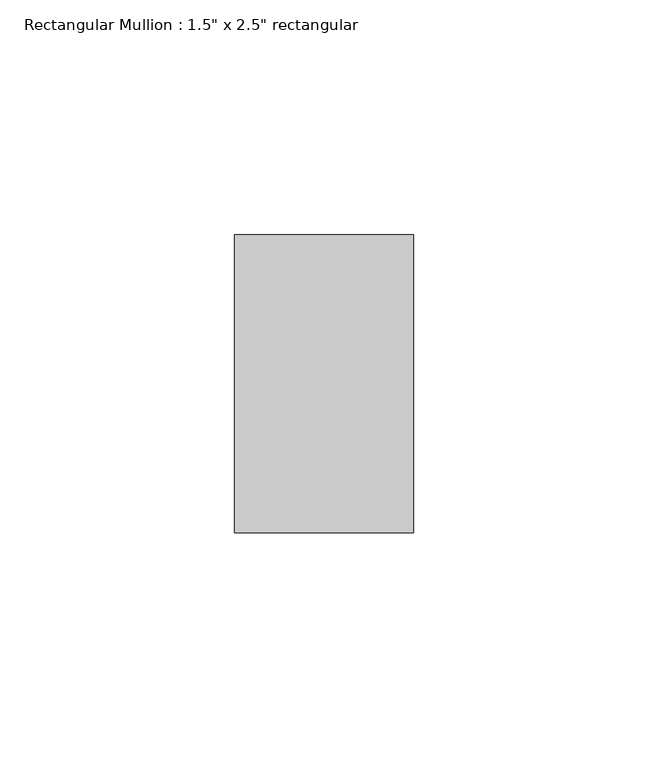
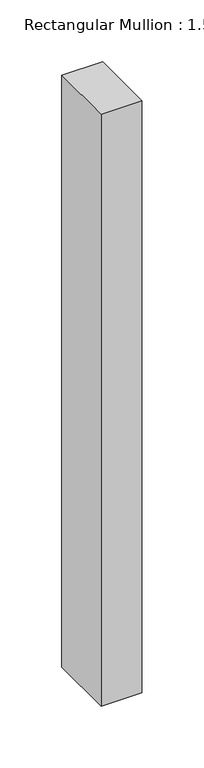
"""IFC4 building model written with IfcOpenShell, lengths in millimetres: member geometry."""

from ifc_helpers import new_model, si_unit, frame, origin, place, context, project, spatial, polyline, outline, extrude, source, transform, mapped, element, save


def member_e8de63ac(model_context):
    return source(origin(), model_context, "Body", "SweptSolid", [
        extrude(outline(polyline([(0.0, 31.75), (0.0, -31.75), (-38.1, -31.75), (-38.1, 31.75), (0.0, 31.75)])), frame((0.0, 0.0, -584.2), z_axis=(0.0, 0.0, 1.0), x_axis=(1.0, 0.0, 0.0)), (0.0, 0.0, 1.0), 584.2),
    ])


if __name__ == "__main__":
    model = new_model("IFC4")
    model_context = context("Model", 3, world=origin())
    ifc_project = project(units=[si_unit("LENGTHUNIT", "METRE", prefix="MILLI")], contexts=[model_context])
    site = spatial("IfcSite", under=ifc_project)
    building = spatial("IfcBuilding", under=site)
    placement = place(None, origin())
    member_shape = member_e8de63ac(model_context)
    element("IfcMember", 1, ObjectType="Rectangular Mullion : 1.5\" x 2.5\" rectangular", at=placement, inside=building, context=model_context, shape_type="MappedRepresentation", body=[
        mapped(member_shape, transform((0.0, 0.0, 0.0), x_axis=(1.0, 0.0, 0.0), y_axis=(0.0, 1.0, 0.0), z_axis=(0.0, 0.0, 1.0))),
    ])
    save(model, "model.ifc")

# Revit data of these elements
# Type "Rectangular Mullion : 1.5\" x 2.5\" rectangular"
#   built-in parameter 1007304 = 0.208333 (stored number, unit not read)
#   built-in parameter 1007301 = 0.0625 (stored number, unit not read)
#   built-in parameter 1007300 = 0.0625 (stored number, unit not read)
# Element 1 (IfcMember, "Rectangular Mullion : 1.5\" x 2.5\" rectangular")
#   Materials on its faces: "Leather - Black"
# Materials
#   "Leather - Black": class "Generic", colour RGB 40 40 40, transparency 0, Cost = 0
